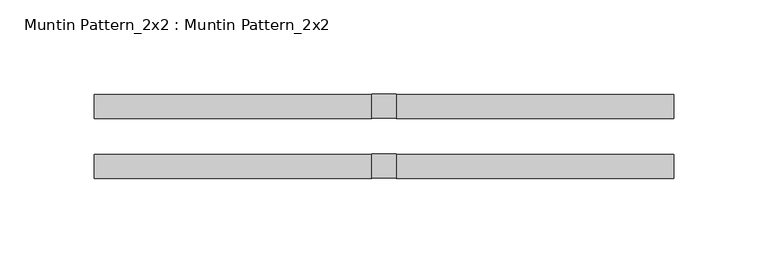
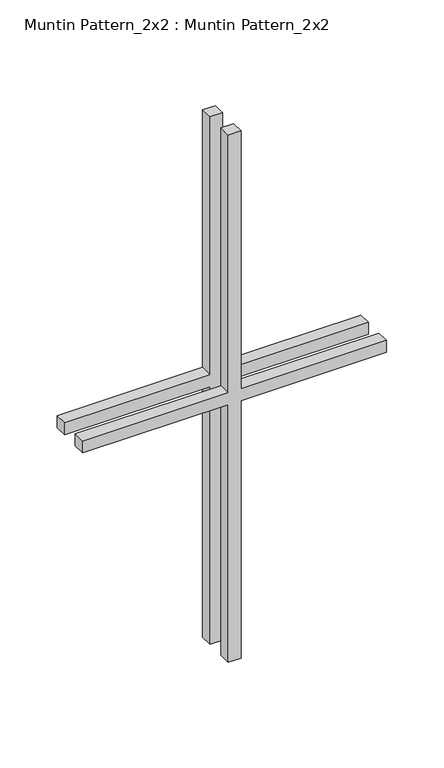
"""IFC4 building model written with IfcOpenShell, lengths in millimetres: proxy geometry, Muntin Pattern_2x2 : Muntin Pattern_2x2."""

from ifc_helpers import new_model, si_unit, frame, origin, place, context, project, spatial, polyline, outline, extrude, source, transform, mapped, element, save


def muntin_pattern_2x2_muntin_pattern_2x2_7c797e2d(model_context):
    return source(origin(), model_context, "Body", "SweptSolid", [
        extrude(outline(polyline([(287.3375, -6.35), (287.3375, -153.19375), (274.6375, -153.19375), (274.6375, -6.35), (0.0, -6.35), (0.0, 6.35), (274.6375, 6.35), (274.6375, 153.19375), (287.3375, 153.19375), (287.3375, 6.35), (561.975, 6.35), (561.975, -6.35), (287.3375, -6.35)])), frame((0.0, -22.225, 0.0), z_axis=(0.0, 1.0, 0.0), x_axis=(0.0, 0.0, 1.0)), (0.0, 0.0, 1.0), 12.7),
        extrude(outline(polyline([(287.3375, -6.35), (287.3375, -153.19375), (274.6375, -153.19375), (274.6375, -6.35), (0.0, -6.35), (0.0, 6.35), (274.6375, 6.35), (274.6375, 153.19375), (287.3375, 153.19375), (287.3375, 6.35), (561.975, 6.35), (561.975, -6.35), (287.3375, -6.35)])), frame((0.0, 9.525, 0.0), z_axis=(0.0, 1.0, 0.0), x_axis=(0.0, 0.0, 1.0)), (0.0, 0.0, 1.0), 12.7),
    ])


if __name__ == "__main__":
    model = new_model("IFC4")
    model_context = context("Model", 3, world=origin())
    ifc_project = project(units=[si_unit("LENGTHUNIT", "METRE", prefix="MILLI")], contexts=[model_context])
    site = spatial("IfcSite", under=ifc_project)
    building = spatial("IfcBuilding", under=site)
    placement = place(None, origin())
    muntin_pattern_2x2_muntin_pattern_2x2_shape = muntin_pattern_2x2_muntin_pattern_2x2_7c797e2d(model_context)
    element("IfcBuildingElementProxy", 1, Name="Muntin Pattern_2x2 : Muntin Pattern_2x2", ObjectType="Muntin Pattern_2x2 : Muntin Pattern_2x2", at=placement, inside=building, context=model_context, shape_type="MappedRepresentation", body=[
        mapped(muntin_pattern_2x2_muntin_pattern_2x2_shape, transform((0.0, 0.0, 0.0), x_axis=(1.0, 0.0, 0.0), y_axis=(0.0, 1.0, 0.0), z_axis=(0.0, 0.0, 1.0))),
    ])
    save(model, "model.ifc")

# Revit data of these elements
# Type "Muntin Pattern_2x2 : Muntin Pattern_2x2"
#   Width [instance default] = 4' - 0"
#   Thickness = 0' - 0 1/2"
#   Height [instance default] = 4' - 0"
#   Distance = 0' - 0 3/4"
#   Interior Material [instance default] = none
#   Exterior Material [instance default] = none
#   Default Elevation = 0
# Element 1 (IfcBuildingElementProxy, "Muntin Pattern_2x2 : Muntin Pattern_2x2")
#   Width = 1' - 0 1/16"
#   Height = 1' - 10 1/8"
#   Interior Material = Wood - Stained
#   Exterior Material = Clad - White
#   Materials on its faces: "Clad - White", "Wood - Stained"
# Materials
#   "Clad - White": class "Wood", colour RGB 242 242 238, transparency 0, Cost = 0
#   "Wood - Stained": class "Wood", colour RGB 224 178 126, transparency 0, Cost = 0
